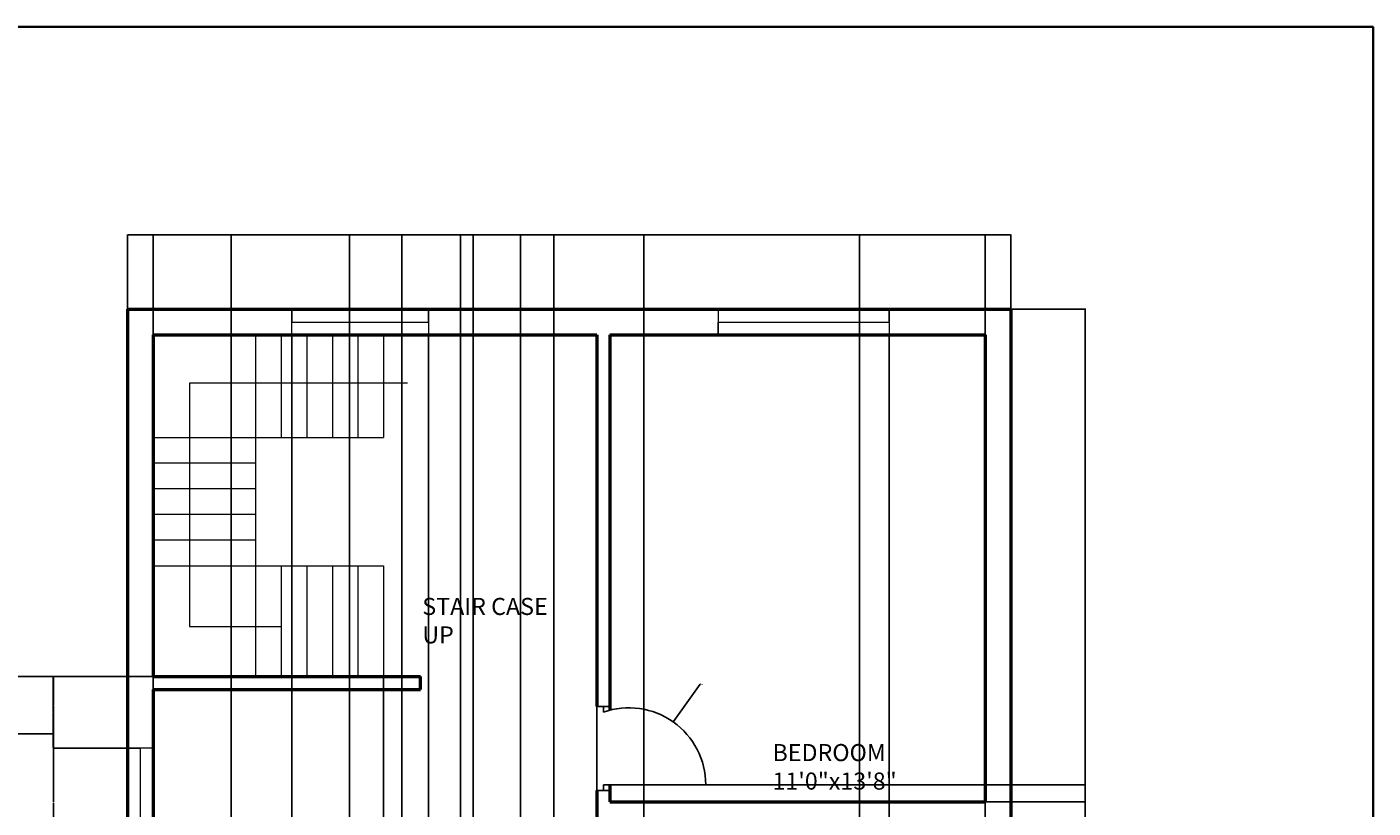
# Model space of a CAD drawing. Units: inches. Extents: x 1860 to 2753, y 1742 to 2419.
# Tile 4 of 4: x 2280 to 2753, y 2145 to 2419. Entities that reach past the tile are written whole.
import ezdxf

# ---------------------------------------------------------------- set-up
doc = ezdxf.new("R2010")
doc.units = ezdxf.units.IN
for name, color, linetype, lineweight in [('A-ANNO-DIMS', 2, 'Continuous', 18), ('A-ANNO-TTLB', 7, 'Continuous', 35), ('A-AREA-IDEN', 7, 'Continuous', 18), ('A-DOOR', 3, 'Continuous', 25), ('A-FLOR-STRS', 7, 'Continuous', 18), ('A-GLAZ', 4, 'Continuous', 18), ('A-WALL', 7, 'Continuous', 50)]:
    doc.layers.add(name, color=color, linetype=linetype, lineweight=lineweight)
doc.styles.get("Standard").update_dxf_attribs({"font": 'arial.ttf'})
doc.dimstyles.get("Standard").update_dxf_attribs({"dimtxt": 0.18, "dimasz": 0.18, "dimexe": 0.18, "dimexo": 0.0625, "dimgap": 0.09, "dimtad": 0, "dimtih": 1, "dimtoh": 1, "dimdec": 4, "dimzin": 0, "dimdsep": 46, "dimtxsty": 'Standard', "dimcen": 0.09, "dimadec": 0, "dimazin": 0, "dimtfac": 1, "dimtdec": 4, "dimtofl": 0, "dimtmove": 0, "dimatfit": 3, "dimfxl": 1, "dimtolj": 1, "dimtzin": 0, "dimarcsym": 0})

# ---------------------------------------------------------------- blocks, each defined once
blk = doc.blocks.new('WIN-60IN')
for p, q in [((0, 9), (0, 0)), ((60, 4.5), (60, 9)), ((60, 9), (60, 0)), ((0, 0), (0, 4.5)), ((0, 4.5), (60, 4.5))]:
    blk.add_line(p, q)
blk = doc.blocks.new('*D20')
at = {"layer": 'A-ANNO-DIMS', "color": 0, "lineweight": -2, "transparency": 16777216}
for p, q in [((2263.53, 2170.97), (2289.75, 2170.97)), ((2289.57, 2170.79), (2289.57, 2147.15)), ((2289.57, 2123.15), (2289.57, 2146.79)), ((2263.53, 2122.97), (2289.75, 2122.97))]:
    blk.add_line(p, q, dxfattribs=at)
at = {"layer": 'A-ANNO-DIMS', "color": 0, "transparency": 16777216}
for points in [[(2289.54, 2170.79), (2289.6, 2170.79), (2289.57, 2170.97)], [(2289.54, 2123.15), (2289.6, 2123.15), (2289.57, 2122.97)]]:
    blk.add_solid(points, dxfattribs=at)
at = {"layer": 'Defpoints', "color": 0, "transparency": 16777216}
for p in [(2263.47, 2170.97), (2289.57, 2170.97), (2263.47, 2122.97)]:
    blk.add_point(p, dxfattribs=at)
at = {"layer": 'A-ANNO-DIMS', "color": 0, "transparency": 16777216, "insert": (2289.57, 2146.97), "char_height": 0.18, "attachment_point": 5}
blk.add_mtext('\\A1;48', dxfattribs=at)
blk = doc.blocks.new('*D21')
at = {"layer": 'A-ANNO-DIMS', "color": 0, "lineweight": -2, "transparency": 16777216}
for p, q in [((2254.53, 2191.15), (2289.75, 2191.15)), ((2289.57, 2190.97), (2289.57, 2181.24)), ((2289.57, 2171.15), (2289.57, 2180.88)), ((2263.53, 2170.97), (2289.75, 2170.97))]:
    blk.add_line(p, q, dxfattribs=at)
at = {"layer": 'A-ANNO-DIMS', "color": 0, "transparency": 16777216}
for points in [[(2289.54, 2190.97), (2289.6, 2190.97), (2289.57, 2191.15)], [(2289.54, 2171.15), (2289.6, 2171.15), (2289.57, 2170.97)]]:
    blk.add_solid(points, dxfattribs=at)
at = {"layer": 'Defpoints', "color": 0, "transparency": 16777216}
for p in [(2254.47, 2191.15), (2289.57, 2191.15), (2263.47, 2170.97)]:
    blk.add_point(p, dxfattribs=at)
at = {"layer": 'A-ANNO-DIMS', "color": 0, "transparency": 16777216, "insert": (2289.57, 2181.06), "char_height": 0.18, "attachment_point": 5}
blk.add_mtext('\\A1;20.18', dxfattribs=at)
blk = doc.blocks.new('*D31')
at = {"layer": 'A-ANNO-DIMS', "color": 0, "lineweight": -2, "transparency": 16777216}
for p, q in [((2315.53, 2320.21), (2315.53, 2346.43)), ((2315.71, 2346.25), (2470.38, 2346.25)), ((2625.85, 2346.25), (2471.17, 2346.25)), ((2626.03, 2320.21), (2626.03, 2346.43))]:
    blk.add_line(p, q, dxfattribs=at)
at = {"layer": 'A-ANNO-DIMS', "color": 0, "transparency": 16777216}
for points in [[(2315.71, 2346.28), (2315.71, 2346.22), (2315.53, 2346.25)], [(2625.85, 2346.28), (2625.85, 2346.22), (2626.03, 2346.25)]]:
    blk.add_solid(points, dxfattribs=at)
at = {"layer": 'Defpoints', "color": 0, "transparency": 16777216}
for p in [(2626.03, 2346.25), (2315.53, 2320.15), (2626.03, 2320.15)]:
    blk.add_point(p, dxfattribs=at)
at = {"layer": 'A-ANNO-DIMS', "color": 0, "transparency": 16777216, "insert": (2470.78, 2346.25), "char_height": 0.18, "attachment_point": 5}
blk.add_mtext('\\A1;310.5', dxfattribs=at)
blk = doc.blocks.new('*D32')
at = {"layer": 'A-ANNO-DIMS', "color": 0, "lineweight": -2, "transparency": 16777216}
for p, q in [((2626.09, 2320.15), (2652.31, 2320.15)), ((2652.13, 2319.97), (2652.13, 2097.33)), ((2652.13, 1874.33), (2652.13, 2096.97)), ((2626.09, 1874.15), (2652.31, 1874.15))]:
    blk.add_line(p, q, dxfattribs=at)
at = {"layer": 'A-ANNO-DIMS', "color": 0, "transparency": 16777216}
for points in [[(2652.1, 2319.97), (2652.16, 2319.97), (2652.13, 2320.15)], [(2652.1, 1874.33), (2652.16, 1874.33), (2652.13, 1874.15)]]:
    blk.add_solid(points, dxfattribs=at)
at = {"layer": 'Defpoints', "color": 0, "transparency": 16777216}
for p in [(2626.03, 2320.15), (2652.13, 2320.15), (2626.03, 1874.15)]:
    blk.add_point(p, dxfattribs=at)
at = {"layer": 'A-ANNO-DIMS', "color": 0, "transparency": 16777216, "insert": (2652.13, 2097.15), "char_height": 0.18, "attachment_point": 5}
blk.add_mtext('\\A1;446', dxfattribs=at)
blk = doc.blocks.new('*D33')
at = {"layer": 'A-ANNO-DIMS', "color": 0, "lineweight": -2, "transparency": 16777216}
for p, q in [((2373.33, 2311.09), (2373.33, 1847.87)), ((2421.33, 2311.09), (2421.33, 1847.87)), ((2373.51, 1848.05), (2397.11, 1848.05)), ((2421.15, 1848.05), (2397.55, 1848.05))]:
    blk.add_line(p, q, dxfattribs=at)
at = {"layer": 'A-ANNO-DIMS', "color": 0, "transparency": 16777216}
for points in [[(2373.51, 1848.08), (2373.51, 1848.02), (2373.33, 1848.05)], [(2421.15, 1848.08), (2421.15, 1848.02), (2421.33, 1848.05)]]:
    blk.add_solid(points, dxfattribs=at)
at = {"layer": 'Defpoints', "color": 0, "transparency": 16777216}
for p in [(2373.33, 2311.15), (2421.33, 2311.15), (2421.33, 1848.05)]:
    blk.add_point(p, dxfattribs=at)
at = {"layer": 'A-ANNO-DIMS', "color": 0, "transparency": 16777216, "insert": (2397.33, 1848.05), "char_height": 0.18, "attachment_point": 5}
blk.add_mtext('\\A1;48', dxfattribs=at)
blk = doc.blocks.new('*D34')
at = {"layer": 'A-ANNO-DIMS', "color": 0, "lineweight": -2, "transparency": 16777216}
for p, q in [((2421.33, 2311.09), (2421.33, 1847.87)), ((2480.53, 2311.09), (2480.53, 1847.87)), ((2421.51, 1848.05), (2450.6, 1848.05)), ((2480.35, 1848.05), (2451.25, 1848.05))]:
    blk.add_line(p, q, dxfattribs=at)
at = {"layer": 'A-ANNO-DIMS', "color": 0, "transparency": 16777216}
for points in [[(2421.51, 1848.08), (2421.51, 1848.02), (2421.33, 1848.05)], [(2480.35, 1848.08), (2480.35, 1848.02), (2480.53, 1848.05)]]:
    blk.add_solid(points, dxfattribs=at)
at = {"layer": 'Defpoints', "color": 0, "transparency": 16777216}
for p in [(2421.33, 2311.15), (2480.53, 2311.15), (2480.53, 1848.05)]:
    blk.add_point(p, dxfattribs=at)
at = {"layer": 'A-ANNO-DIMS', "color": 0, "transparency": 16777216, "insert": (2450.93, 1848.05), "char_height": 0.18, "attachment_point": 5}
blk.add_mtext('\\A1;59.2', dxfattribs=at)
blk = doc.blocks.new('*D35')
at = {"layer": 'A-ANNO-DIMS', "color": 0, "lineweight": -2, "transparency": 16777216}
for p, q in [((2583.19, 2311.09), (2583.19, 1847.87)), ((2617.03, 2311.09), (2617.03, 1847.87)), ((2583.37, 1848.05), (2599.71, 1848.05)), ((2616.85, 1848.05), (2600.5, 1848.05))]:
    blk.add_line(p, q, dxfattribs=at)
at = {"layer": 'A-ANNO-DIMS', "color": 0, "transparency": 16777216}
for points in [[(2583.37, 1848.08), (2583.37, 1848.02), (2583.19, 1848.05)], [(2616.85, 1848.08), (2616.85, 1848.02), (2617.03, 1848.05)]]:
    blk.add_solid(points, dxfattribs=at)
at = {"layer": 'Defpoints', "color": 0, "transparency": 16777216}
for p in [(2583.19, 2311.15), (2617.03, 2311.15), (2617.03, 1848.05)]:
    blk.add_point(p, dxfattribs=at)
at = {"layer": 'A-ANNO-DIMS', "color": 0, "transparency": 16777216, "insert": (2600.11, 1848.05), "char_height": 0.18, "attachment_point": 5}
blk.add_mtext('\\A1;33.84', dxfattribs=at)
blk = doc.blocks.new('*D36')
at = {"layer": 'A-ANNO-DIMS', "color": 0, "lineweight": -2, "transparency": 16777216}
for p, q in [((2324.53, 1946.21), (2324.53, 2346.43)), ((2324.71, 2346.25), (2337.76, 2346.25)), ((2351.74, 2346.25), (2338.69, 2346.25)), ((2351.92, 1946.21), (2351.92, 2346.43))]:
    blk.add_line(p, q, dxfattribs=at)
at = {"layer": 'A-ANNO-DIMS', "color": 0, "transparency": 16777216}
for points in [[(2324.71, 2346.28), (2324.71, 2346.22), (2324.53, 2346.25)], [(2351.74, 2346.28), (2351.74, 2346.22), (2351.92, 2346.25)]]:
    blk.add_solid(points, dxfattribs=at)
at = {"layer": 'Defpoints', "color": 0, "transparency": 16777216}
for p in [(2351.92, 2346.25), (2324.53, 1946.15), (2351.92, 1946.15)]:
    blk.add_point(p, dxfattribs=at)
at = {"layer": 'A-ANNO-DIMS', "color": 0, "transparency": 16777216, "insert": (2338.22, 2346.25), "char_height": 0.18, "attachment_point": 5}
blk.add_mtext('\\A1;27.396', dxfattribs=at)
blk = doc.blocks.new('*D37')
at = {"layer": 'A-ANNO-DIMS', "color": 0, "lineweight": -2, "transparency": 16777216}
for p, q in [((2411.92, 1946.21), (2411.92, 2346.43)), ((2412.1, 2346.25), (2421.76, 2346.25)), ((2432.35, 2346.25), (2422.69, 2346.25)), ((2432.53, 1946.21), (2432.53, 2346.43))]:
    blk.add_line(p, q, dxfattribs=at)
at = {"layer": 'A-ANNO-DIMS', "color": 0, "transparency": 16777216}
for points in [[(2412.1, 2346.28), (2412.1, 2346.22), (2411.92, 2346.25)], [(2432.35, 2346.28), (2432.35, 2346.22), (2432.53, 2346.25)]]:
    blk.add_solid(points, dxfattribs=at)
at = {"layer": 'Defpoints', "color": 0, "transparency": 16777216}
for p in [(2432.53, 2346.25), (2411.92, 1946.15), (2432.53, 1946.15)]:
    blk.add_point(p, dxfattribs=at)
at = {"layer": 'A-ANNO-DIMS', "color": 0, "transparency": 16777216, "insert": (2422.22, 2346.25), "char_height": 0.18, "attachment_point": 5}
blk.add_mtext('\\A1;20.604', dxfattribs=at)
blk = doc.blocks.new('*D42')
at = {"layer": 'A-ANNO-DIMS', "color": 0, "lineweight": -2, "transparency": 16777216}
for p, q in [((2324.46, 2191.15), (2289.25, 2191.15)), ((2289.43, 2190.97), (2289.43, 2178.75)), ((2289.43, 2166.17), (2289.43, 2178.39)), ((2315.46, 2165.99), (2289.25, 2165.99))]:
    blk.add_line(p, q, dxfattribs=at)
at = {"layer": 'A-ANNO-DIMS', "color": 0, "transparency": 16777216}
for points in [[(2289.4, 2190.97), (2289.46, 2190.97), (2289.43, 2191.15)], [(2289.4, 2166.17), (2289.46, 2166.17), (2289.43, 2165.99)]]:
    blk.add_solid(points, dxfattribs=at)
at = {"layer": 'Defpoints', "color": 0, "transparency": 16777216}
for p in [(2289.43, 2191.15), (2324.53, 2191.15), (2315.53, 2165.99)]:
    blk.add_point(p, dxfattribs=at)
at = {"layer": 'A-ANNO-DIMS', "color": 0, "transparency": 16777216, "insert": (2289.43, 2178.57), "char_height": 0.18, "attachment_point": 5}
blk.add_mtext('\\A1;25.16', dxfattribs=at)
blk = doc.blocks.new('*D43')
at = {"layer": 'A-ANNO-DIMS', "color": 0, "lineweight": -2, "transparency": 16777216}
for p, q in [((2437.03, 1946.21), (2437.03, 2346.43)), ((2437.21, 2346.25), (2444.97, 2346.25)), ((2453.51, 2346.25), (2445.74, 2346.25)), ((2453.69, 1946.21), (2453.69, 2346.43))]:
    blk.add_line(p, q, dxfattribs=at)
at = {"layer": 'A-ANNO-DIMS', "color": 0, "transparency": 16777216}
for points in [[(2437.21, 2346.28), (2437.21, 2346.22), (2437.03, 2346.25)], [(2453.51, 2346.28), (2453.51, 2346.22), (2453.69, 2346.25)]]:
    blk.add_solid(points, dxfattribs=at)
at = {"layer": 'Defpoints', "color": 0, "transparency": 16777216}
for p in [(2453.69, 2346.25), (2437.03, 1946.15), (2453.69, 1946.15)]:
    blk.add_point(p, dxfattribs=at)
at = {"layer": 'A-ANNO-DIMS', "color": 0, "transparency": 16777216, "insert": (2445.36, 2346.25), "char_height": 0.18, "attachment_point": 5}
blk.add_mtext('\\A1;16.67', dxfattribs=at)
blk = doc.blocks.new('*D44')
at = {"layer": 'A-ANNO-DIMS', "color": 0, "lineweight": -2, "transparency": 16777216}
for p, q in [((2572.85, 1946.21), (2572.85, 2346.43)), ((2573.03, 2346.25), (2594.54, 2346.25)), ((2616.85, 2346.25), (2595.34, 2346.25)), ((2617.03, 1946.21), (2617.03, 2346.43))]:
    blk.add_line(p, q, dxfattribs=at)
at = {"layer": 'A-ANNO-DIMS', "color": 0, "transparency": 16777216}
for points in [[(2573.03, 2346.28), (2573.03, 2346.22), (2572.85, 2346.25)], [(2616.85, 2346.28), (2616.85, 2346.22), (2617.03, 2346.25)]]:
    blk.add_solid(points, dxfattribs=at)
at = {"layer": 'Defpoints', "color": 0, "transparency": 16777216}
for p in [(2617.03, 2346.25), (2572.85, 1946.15), (2617.03, 1946.15)]:
    blk.add_point(p, dxfattribs=at)
at = {"layer": 'A-ANNO-DIMS', "color": 0, "transparency": 16777216, "insert": (2594.94, 2346.25), "char_height": 0.18, "attachment_point": 5}
blk.add_mtext('\\A1;44.17', dxfattribs=at)
blk = doc.blocks.new('*D46')
at = {"layer": 'A-ANNO-DIMS', "color": 0, "lineweight": -2, "transparency": 16777216}
for p, q in [((2324.53, 2066.21), (2324.53, 2346.43)), ((2324.71, 2346.25), (2358.67, 2346.25)), ((2393.43, 2346.25), (2359.46, 2346.25)), ((2393.61, 2066.21), (2393.61, 2346.43))]:
    blk.add_line(p, q, dxfattribs=at)
at = {"layer": 'A-ANNO-DIMS', "color": 0, "transparency": 16777216}
for points in [[(2324.71, 2346.28), (2324.71, 2346.22), (2324.53, 2346.25)], [(2393.43, 2346.28), (2393.43, 2346.22), (2393.61, 2346.25)]]:
    blk.add_solid(points, dxfattribs=at)
at = {"layer": 'Defpoints', "color": 0, "transparency": 16777216}
for p in [(2393.61, 2346.25), (2324.53, 2066.15), (2393.61, 2066.15)]:
    blk.add_point(p, dxfattribs=at)
at = {"layer": 'A-ANNO-DIMS', "color": 0, "transparency": 16777216, "insert": (2359.07, 2346.25), "char_height": 0.18, "attachment_point": 5}
blk.add_mtext('\\A1;69.08', dxfattribs=at)
blk = doc.blocks.new('*D47')
at = {"layer": 'A-ANNO-DIMS', "color": 0, "lineweight": -2, "transparency": 16777216}
for p, q in [((2405.53, 2191.09), (2405.53, 1847.87)), ((2324.53, 2186.59), (2324.53, 1847.87)), ((2324.71, 1848.05), (2364.82, 1848.05)), ((2405.35, 1848.05), (2365.23, 1848.05))]:
    blk.add_line(p, q, dxfattribs=at)
at = {"layer": 'A-ANNO-DIMS', "color": 0, "transparency": 16777216}
for points in [[(2324.71, 1848.08), (2324.71, 1848.02), (2324.53, 1848.05)], [(2405.35, 1848.08), (2405.35, 1848.02), (2405.53, 1848.05)]]:
    blk.add_solid(points, dxfattribs=at)
at = {"layer": 'Defpoints', "color": 0, "transparency": 16777216}
for p in [(2405.53, 2191.15), (2324.53, 2186.65), (2405.53, 1848.05)]:
    blk.add_point(p, dxfattribs=at)
at = {"layer": 'A-ANNO-DIMS', "color": 0, "transparency": 16777216, "insert": (2365.03, 1848.05), "char_height": 0.18, "attachment_point": 5}
blk.add_mtext('\\A1;81', dxfattribs=at)
blk = doc.blocks.new('*D48')
at = {"layer": 'A-ANNO-DIMS', "color": 0, "lineweight": -2, "transparency": 16777216}
for p, q in [((2465.35, 2034.71), (2465.35, 2346.43)), ((2465.53, 2346.25), (2480.8, 2346.25)), ((2496.85, 2346.25), (2481.58, 2346.25)), ((2497.03, 2034.71), (2497.03, 2346.43))]:
    blk.add_line(p, q, dxfattribs=at)
at = {"layer": 'A-ANNO-DIMS', "color": 0, "transparency": 16777216}
for points in [[(2465.53, 2346.28), (2465.53, 2346.22), (2465.35, 2346.25)], [(2496.85, 2346.28), (2496.85, 2346.22), (2497.03, 2346.25)]]:
    blk.add_solid(points, dxfattribs=at)
at = {"layer": 'Defpoints', "color": 0, "transparency": 16777216}
for p in [(2497.03, 2346.25), (2465.35, 2034.65), (2497.03, 2034.65)]:
    blk.add_point(p, dxfattribs=at)
at = {"layer": 'A-ANNO-DIMS', "color": 0, "transparency": 16777216, "insert": (2481.19, 2346.25), "char_height": 0.18, "attachment_point": 5}
blk.add_mtext('\\A1;31.67', dxfattribs=at)
blk = doc.blocks.new('*D50')
at = {"layer": 'A-ANNO-DIMS', "color": 0, "lineweight": -2, "transparency": 16777216}
for p, q in [((2485.09, 2153.12), (2652.31, 2153.12)), ((2652.13, 2152.94), (2652.13, 2150.31)), ((2652.13, 2147.33), (2652.13, 2149.95)), ((2485.09, 2147.15), (2652.31, 2147.15))]:
    blk.add_line(p, q, dxfattribs=at)
at = {"layer": 'A-ANNO-DIMS', "color": 0, "transparency": 16777216}
for points in [[(2652.1, 2152.94), (2652.16, 2152.94), (2652.13, 2153.12)], [(2652.1, 2147.33), (2652.16, 2147.33), (2652.13, 2147.15)]]:
    blk.add_solid(points, dxfattribs=at)
at = {"layer": 'Defpoints', "color": 0, "transparency": 16777216}
for p in [(2485.03, 2153.12), (2652.13, 2153.12), (2485.03, 2147.15)]:
    blk.add_point(p, dxfattribs=at)
at = {"layer": 'A-ANNO-DIMS', "color": 0, "transparency": 16777216, "insert": (2652.13, 2150.13), "char_height": 0.18, "attachment_point": 5}
blk.add_mtext('\\A1;5.97', dxfattribs=at)
blk = doc.blocks.new('*D57')
at = {"layer": 'A-ANNO-DIMS', "color": 0, "lineweight": -2, "transparency": 16777216}
for p, q in [((2516.76, 2188.42), (2507.48, 2175.33)), ((2516.94, 2188.42), (2516.76, 2188.42)), ((2491.64, 2153.12), (2491.82, 2153.12)), ((2491.73, 2153.03), (2491.73, 2153.21))]:
    blk.add_line(p, q, dxfattribs=at)
at = {"layer": 'A-ANNO-DIMS', "color": 0, "transparency": 16777216}
blk.add_solid([(2507.45, 2175.35), (2507.5, 2175.31), (2507.37, 2175.18)], dxfattribs=at)
at = {"layer": 'Defpoints', "color": 0, "transparency": 16777216}
for p in [(2507.37, 2175.18), (2491.73, 2153.12)]:
    blk.add_point(p, dxfattribs=at)
at = {"layer": 'A-ANNO-DIMS', "color": 0, "transparency": 16777216, "insert": (2517.42, 2188.42), "char_height": 0.18, "attachment_point": 5}
blk.add_mtext('\\A1;R27.05', dxfattribs=at)

msp = doc.modelspace()

# ---------------------------------------------------------------- linework, layer by layer
at = {"layer": 'A-ANNO-TTLB'}
msp.add_lwpolyline([(1859.5561, 2419.29), (2753.3204, 2419.29), (2753.3204, 1741.6035), (1859.5561, 1741.6035)], close=True, dxfattribs=at)
at = {"layer": 'A-DOOR'}
for p, q in [((2480.525, 2180.6432), (2485.025, 2180.6432)), ((2485.025, 2180.6432), (2482.775, 2180.6432)), ((2482.775, 2180.6432), (2482.775, 2178.6432)), ((2482.775, 2151.1172), (2482.775, 2153.1172)), ((2482.775, 2153.1172), (2518.775, 2153.1172)), ((2480.525, 2151.1172), (2485.025, 2151.1172)), ((2485.025, 2151.1172), (2482.775, 2151.1172))]:
    msp.add_line(p, q, dxfattribs=at)
msp.add_arc((2491.7253, 2153.1172), 27.0497, 0, 109.322407, dxfattribs=at)
at = {"layer": 'A-FLOR-STRS'}
for p, q in [((2324.525, 2311.1476), (2360.525, 2311.1476)), ((2360.525, 2311.1476), (2360.525, 2275.1476)), ((2369.525, 2311.1476), (2369.525, 2275.1476)), ((2378.525, 2311.1476), (2378.525, 2275.1476)), ((2387.525, 2311.1476), (2387.525, 2275.1476)), ((2396.525, 2311.1476), (2396.525, 2275.1476)), ((2405.525, 2311.1476), (2405.525, 2275.1476)), ((2413.9312, 2294.1746), (2337.3116, 2294.1746)), ((2337.3116, 2294.1746), (2337.3116, 2208.7459)), ((2324.525, 2275.1476), (2405.525, 2275.1476)), ((2360.525, 2275.1476), (2360.525, 2239.1476)), ((2324.525, 2266.1476), (2360.525, 2266.1476)), ((2324.525, 2257.1476), (2360.525, 2257.1476)), ((2324.525, 2248.1476), (2360.525, 2248.1476)), ((2324.525, 2239.1476), (2360.525, 2239.1476)), ((2360.525, 2239.1476), (2360.525, 2203.1476)), ((2324.525, 2229.9769), (2405.525, 2229.9769)), ((2369.525, 2229.9769), (2369.525, 2203.1476)), ((2378.525, 2229.9769), (2378.525, 2191.1476)), ((2387.525, 2229.9769), (2387.525, 2191.1476)), ((2396.525, 2229.9769), (2396.525, 2191.1476)), ((2405.525, 2229.9769), (2405.525, 2191.1476)), ((2337.3116, 2208.7459), (2369.525, 2208.7459)), ((2360.525, 2203.1476), (2360.525, 2191.1476)), ((2369.525, 2203.1476), (2369.525, 2191.1476))]:
    msp.add_line(p, q, dxfattribs=at)
at = {"layer": 'A-GLAZ'}
for p, q in [((2373.3292, 2311.1476), (2373.3292, 2320.1476)), ((2373.3292, 2320.1476), (2373.3292, 2315.6476)), ((2421.3292, 2315.6476), (2421.3292, 2320.1476)), ((2421.3292, 2320.1476), (2421.3292, 2311.1476)), ((2373.3292, 2315.6476), (2421.3292, 2315.6476))]:
    msp.add_line(p, q, dxfattribs=at)
at = {"layer": 'A-WALL'}
for p, q in [((2315.525, 2320.1476), (2626.025, 2320.1476)), ((2315.525, 2320.1476), (2315.525, 1937.1476)), ((2626.025, 2320.1476), (2626.025, 1874.1476)), ((2324.525, 2311.1476), (2480.525, 2311.1476)), ((2324.525, 2311.1476), (2324.525, 2191.1476)), ((2480.525, 2311.1476), (2480.525, 2180.6432)), ((2485.025, 2311.1476), (2485.025, 2179.3239)), ((2485.025, 2311.1476), (2617.025, 2311.1476)), ((2617.025, 2311.1476), (2617.025, 2147.1476)), ((2324.525, 2191.1476), (2418.4699, 2191.1476)), ((2418.4699, 2186.6476), (2418.4699, 2191.1476)), ((2324.525, 2186.6476), (2418.4699, 2186.6476)), ((2324.525, 2186.6476), (2324.525, 2070.6476)), ((2485.025, 2153.1172), (2485.025, 2147.1476)), ((2480.525, 2151.1172), (2480.525, 2103.664)), ((2485.025, 2147.1476), (2617.025, 2147.1476))]:
    msp.add_line(p, q, dxfattribs=at)

# ---------------------------------------------------------------- block references
at = {"layer": 'A-GLAZ'}
msp.add_blockref('WIN-60IN', (2523.1855, 2311.1476), dxfattribs=at)
at = {"layer": 'A-GLAZ', "rotation": 270.0000000000017}
msp.add_blockref('WIN-60IN', (2315.525, 2165.9892), dxfattribs=at)

# ---------------------------------------------------------------- texts
at = {"layer": 'A-AREA-IDEN', "char_height": 6, "attachment_point": 1}
for s, width, insert in [('STAIR CASE\\PUP', 91.896879, (2419.1468, 2218.7655)), ('BEDROOM\\P11\'0"x13\'8"', 100.432571, (2542.2277, 2167.4318))]:
    msp.add_mtext_dynamic_manual_height_columns(s, width=width, gutter_width=12.5, heights=[0], dxfattribs=dict(at, insert=insert))

# ---------------------------------------------------------------- dimensions: what is measured, and where the dimension line sits
at = {"layer": 'A-ANNO-DIMS'}
for base, p1, p2, override, picture, middle in [((2626.025, 2346.2476), (2315.525, 2320.1476), (2626.025, 2320.1476), {"dimdec": 1, "dimlfac": 1, "dimrnd": 0, "dimzin": 0, "dimdsep": 46, "dimlunit": 2}, '*D31', (2470.775, 2346.2476)), ((2351.9209, 2346.2476), (2324.525, 1946.1476), (2351.9209, 1946.1476), {"dimdec": 3, "dimlfac": 1, "dimrnd": 0, "dimzin": 0, "dimdsep": 46, "dimlunit": 2}, '*D36', (2338.223, 2346.2476)), ((2393.6072, 2346.2476), (2324.525, 2066.1476), (2393.6072, 2066.1476), {"dimdec": 2, "dimlfac": 1, "dimrnd": 0, "dimzin": 0, "dimdsep": 46, "dimlunit": 2}, '*D46', (2359.0661, 2346.2476)), ((2432.525, 2346.2476), (2411.9209, 1946.1476), (2432.525, 1946.1476), {"dimdec": 3, "dimlfac": 1, "dimrnd": 0, "dimzin": 0, "dimdsep": 46, "dimlunit": 2}, '*D37', (2422.223, 2346.2476)), ((2453.6944, 2346.2476), (2437.025, 1946.1476), (2453.6944, 1946.1476), {"dimdec": 2, "dimlfac": 1, "dimrnd": 0, "dimzin": 0, "dimdsep": 46, "dimlunit": 2}, '*D43', (2445.3597, 2346.2476)), ((2497.025, 2346.2476), (2465.355, 2034.6476), (2497.025, 2034.6476), {"dimdec": 2, "dimlfac": 1, "dimrnd": 0, "dimzin": 0, "dimdsep": 46, "dimlunit": 2}, '*D48', (2481.19, 2346.2476)), ((2617.025, 2346.2476), (2572.854, 1946.1476), (2617.025, 1946.1476), {"dimdec": 2, "dimlfac": 1, "dimrnd": 0, "dimzin": 0, "dimdsep": 46, "dimlunit": 2}, '*D44', (2594.9395, 2346.2476)), ((2421.3292, 1848.0476), (2373.3292, 2311.1476), (2421.3292, 2311.1476), {"dimdec": 0, "dimlfac": 1, "dimrnd": 0, "dimzin": 0, "dimdsep": 46, "dimlunit": 2}, '*D33', (2397.3292, 1848.0476)), ((2480.525, 1848.0476), (2421.3292, 2311.1476), (2480.525, 2311.1476), {"dimdec": 1, "dimlfac": 1, "dimrnd": 0, "dimzin": 0, "dimdsep": 46, "dimlunit": 2}, '*D34', (2450.9271, 1848.0476)), ((2617.025, 1848.0476), (2583.1855, 2311.1476), (2617.025, 2311.1476), {"dimdec": 2, "dimlfac": 1, "dimrnd": 0, "dimzin": 0, "dimdsep": 46, "dimlunit": 2}, '*D35', (2600.1053, 1848.0476)), ((2405.525, 1848.0476), (2324.525, 2186.6476), (2405.525, 2191.1476), {"dimdec": 0, "dimlfac": 1, "dimrnd": 0, "dimzin": 0, "dimdsep": 46, "dimlunit": 2}, '*D47', (2365.025, 1848.0476))]:
    dim = msp.add_linear_dim(base=base, p1=p1, p2=p2, dimstyle='Standard', override=override, dxfattribs=at)
    dim.commit()
    dim.dimension.update_dxf_attribs({"geometry": picture, "text_midpoint": middle})
for base, p1, p2, override, picture, middle in [((2652.125, 2320.1476), (2626.025, 1874.1476), (2626.025, 2320.1476), {"dimdec": 0, "dimlfac": 1, "dimrnd": 0, "dimzin": 0, "dimdsep": 46, "dimlunit": 2}, '*D32', (2652.125, 2097.1476)), ((2289.5703, 2191.1476), (2263.4703, 2170.9674), (2254.4703, 2191.1476), {"dimdec": 2, "dimlfac": 1, "dimrnd": 0, "dimzin": 0, "dimdsep": 46, "dimlunit": 2}, '*D21', (2289.5703, 2181.0575)), ((2289.425, 2191.1476), (2315.525, 2165.9892), (2324.525, 2191.1476), {"dimdec": 2, "dimlfac": 1, "dimrnd": 0, "dimzin": 0, "dimdsep": 46, "dimlunit": 2}, '*D42', (2289.425, 2178.5684)), ((2289.5703, 2170.9674), (2263.4703, 2122.9674), (2263.4703, 2170.9674), {"dimdec": 0, "dimlfac": 1, "dimrnd": 0, "dimzin": 0, "dimdsep": 46, "dimlunit": 2}, '*D20', (2289.5703, 2146.9674)), ((2652.125, 2153.1172), (2485.025, 2147.1476), (2485.025, 2153.1172), {"dimdec": 2, "dimlfac": 1, "dimrnd": 0, "dimzin": 0, "dimdsep": 46, "dimlunit": 2}, '*D50', (2652.125, 2150.1324))]:
    dim = msp.add_linear_dim(base=base, p1=p1, p2=p2, angle=90, dimstyle='Standard', override=override, dxfattribs=at)
    dim.commit()
    dim.dimension.update_dxf_attribs({"geometry": picture, "text_midpoint": middle})
dim = msp.add_radius_dim(center=(2491.7253, 2153.1172), mpoint=(2507.371, 2175.183), dimstyle='Standard', override={"dimdec": 2, "dimlfac": 1, "dimrnd": 0, "dimzin": 0, "dimdsep": 46, "dimlunit": 2}, dxfattribs=at)
dim.commit()
dim.dimension.update_dxf_attribs({"geometry": '*D57', "text_midpoint": (2517.4189, 2188.4225), "dimtype": 164})

doc.saveas('drawing.dxf')
